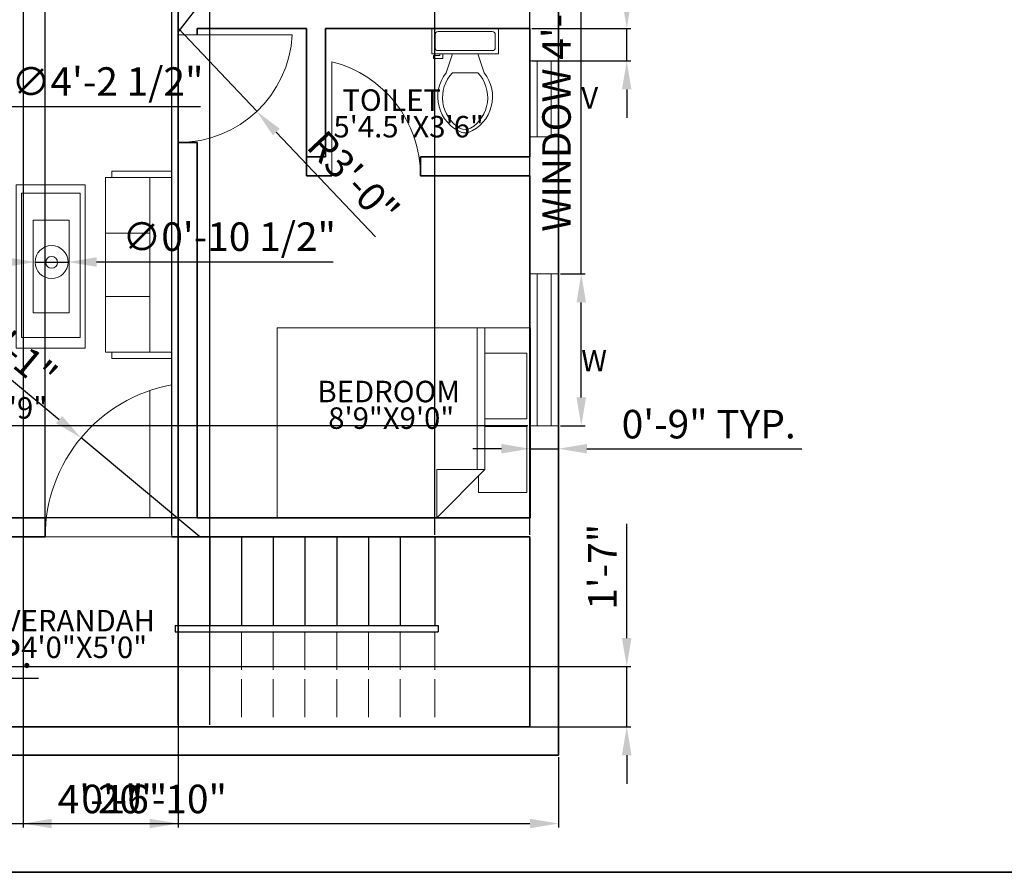
# Model space of a CAD drawing. Units: inches. Extents: x 1838 to 3181, y 1882 to 2430.
# Tile 2 of 4: x 2073 to 2384, y 1894 to 2163. Entities that reach past the tile are written whole.
import ezdxf

# ---------------------------------------------------------------- set-up
doc = ezdxf.new("R2010")
doc.units = ezdxf.units.IN
doc.linetypes.add('ACAD_ISO02W100', pattern=[15, 12, -3])
for name, color, linetype, lineweight in [('A-ANNO-TEXT', 7, 'Continuous', 18), ('A-ANNO-TTLB', 7, 'Continuous', 35), ('A-AREA-IDEN', 7, 'Continuous', 18), ('A-DOOR', 4, 'Continuous', 18), ('A-FLOR-FIXT', 9, 'Continuous', 18), ('A-FLOR-STRS', 7, 'Continuous', 25), ('A-FLOR-STRS-HIDN', 7, 'ACAD_ISO02W100', 18), ('A-FURN', 8, 'Continuous', 18), ('A-GLAZ', 11, 'Continuous', 18), ('A-WALL', 7, 'Continuous', 35), ('S-ANNO-DIMS', 2, 'Continuous', 18)]:
    doc.layers.add(name, color=color, linetype=linetype, lineweight=lineweight)
doc.styles.get("Standard").update_dxf_attribs({"font": 'arial.ttf'})
doc.dimstyles.new('ISO-25', dxfattribs={"dimtxt": 9, "dimasz": 9, "dimexe": 1.25, "dimexo": 0.625, "dimgap": 2, "dimtad": 1, "dimdec": 1, "dimlunit": 4, "dimtxsty": 'Standard', "dimcen": 2.5, "dimadec": 0, "dimazin": 0, "dimtfac": 1, "dimtdec": 1, "dimtmove": 0, "dimatfit": 3, "dimfxl": 1, "dimarcsym": 0})

# ---------------------------------------------------------------- blocks, each defined once
blk = doc.blocks.new('Bed - Queen')
for p, q in [((0, -80.00003), (0, 0)), ((0, 0), (59.99999, 0)), ((59.99999, 0), (59.99999, -80.00003)), ((7.99999, -1.2), (28.79998, -1.2)), ((7.99999, -14.4), (7.99999, -1.2)), ((28.79998, -1.2), (28.79998, -14.4)), ((31.19999, -1.2), (51.99999, -1.2)), ((31.19999, -14.4), (31.19999, -1.2)), ((51.99999, -1.2), (51.99999, -16.4)), ((0, -14.4), (44.8, -14.4)), ((59.99999, -29.6), (44.8, -14.4)), ((44.8, -14.4), (44.8, -29.6)), ((44.8, -16.8), (0, -16.8)), ((51.99999, -16.4), (46.79936, -16.4)), ((44.8, -29.6), (59.99999, -29.6)), ((59.99999, -80.00003), (0, -80.00003))]:
    blk.add_line(p, q)
blk = doc.blocks.new('Toilet - top')
for p, q in [((9.5, -6), (9.5, -2)), ((-10, -8.5), (-8, -8.5)), ((-10, -9.5), (-10, -8.5)), ((-8, -8.5), (-8, -8)), ((-7, -8), (-7, -9.5)), ((-4, -8), (-6, -14)), ((4, -8), (6, -14)), ((-7, -9.5), (-10, -9.5)), ((4, -14), (-4, -14))]:
    blk.add_line(p, q)
blk.add_lwpolyline([(10.5, -8), (10.5, 0), (-10.5, 0), (-10.5, -8)], close=True)
for points in [[(-9.5, -2), (-9.5, -6)], [(8.5, -1), (-8.5, -1)], [(-8.5, -7), (8.5, -7)]]:
    blk.add_lwpolyline(points)
for centre, radius, start, end in [((-8.62, -1.88), 0.884, 81.8699, 188.1301), ((8.62, -1.88), 0.884, 351.8699, 98.1301), ((-8.62, -6.12), 0.884, 171.8699, 278.1301), ((8.62, -6.12), 0.884, 261.8699, 8.1301), ((3.52, -21.58), 12.17, 141.4691, 247.9714), ((4.2, -21.82), 11.33, 136.3677, 238.9468), ((-3.52, -21.58), 12.17, 292.0284, 38.5307), ((-4.2, -21.82), 11.33, 301.053, 43.6321), ((0, -27.88), 4, 245.7318, 294.2682), ((0, -29), 4, 254.8605, 285.1395)]:
    blk.add_arc(centre, radius, start, end)
blk = doc.blocks.new('WIN-48')
for p, q in [((0, 48), (9, 48)), ((2.25, 48), (2.25, 0)), ((6.75, 48), (6.75, 0)), ((0, 0), (9, 0))]:
    blk.add_line(p, q)
blk = doc.blocks.new('VENT-24')
for p, q in [((0, 24), (9, 24)), ((2.25, 24), (2.25, 0)), ((6.75, 24), (6.75, 0)), ((0, 0), (9, 0))]:
    blk.add_line(p, q)
blk = doc.blocks.new('DOOR-SWING-36')
blk.add_line((0, 0), (36, 0))
blk.add_arc((0, -9.14), 37.14, 14.25, 90)
blk = doc.blocks.new('*D23')
at = {"layer": 'Defpoints', "color": 0, "transparency": 16777216}
for p in [(2243.53, 2082.46), (2250.73, 2082.46), (2243.53, 2034.46)]:
    blk.add_point(p, dxfattribs=at)
at = {"layer": 'S-ANNO-DIMS', "color": 0, "lineweight": -2, "transparency": 16777216}
for p, q in [((2250.73, 2082.46), (2250.73, 2209.34)), ((2244.16, 2082.46), (2251.98, 2082.46)), ((2250.73, 2043.46), (2250.73, 2073.46)), ((2244.16, 2034.46), (2251.98, 2034.46))]:
    blk.add_line(p, q, dxfattribs=at)
at = {"layer": 'S-ANNO-DIMS', "color": 0, "transparency": 16777216}
for points in [[(2249.23, 2073.46), (2252.23, 2073.46), (2250.73, 2082.46)], [(2249.23, 2043.46), (2252.23, 2043.46), (2250.73, 2034.46)]]:
    blk.add_solid(points, dxfattribs=at)
at = {"layer": 'S-ANNO-DIMS', "color": 0, "transparency": 16777216, "insert": (2244.08, 2150.4), "char_height": 9, "attachment_point": 5, "rotation": 90}
blk.add_mtext('WINDOW 4\'-0" TYP.', dxfattribs=at)
blk = doc.blocks.new('*D24')
at = {"layer": 'Defpoints', "color": 0, "transparency": 16777216}
for p in [(2234.53, 2034.46), (2243.53, 2034.46), (2243.53, 2027.26)]:
    blk.add_point(p, dxfattribs=at)
at = {"layer": 'S-ANNO-DIMS', "color": 0, "lineweight": -2, "transparency": 16777216}
for p, q in [((2234.53, 2033.83), (2234.53, 2026.01)), ((2243.53, 2033.83), (2243.53, 2026.01)), ((2225.53, 2027.26), (2216.53, 2027.26)), ((2234.53, 2027.26), (2243.53, 2027.26)), ((2252.53, 2027.26), (2320.39, 2027.26))]:
    blk.add_line(p, q, dxfattribs=at)
at = {"layer": 'S-ANNO-DIMS', "color": 0, "transparency": 16777216}
for points in [[(2225.53, 2028.76), (2225.53, 2025.76), (2234.53, 2027.26)], [(2252.53, 2028.76), (2252.53, 2025.76), (2243.53, 2027.26)]]:
    blk.add_solid(points, dxfattribs=at)
at = {"layer": 'S-ANNO-DIMS', "color": 0, "transparency": 16777216, "insert": (2290.96, 2033.85), "char_height": 9, "attachment_point": 5}
blk.add_mtext('0\'-9" TYP.', dxfattribs=at)
blk = doc.blocks.new('*D26')
at = {"layer": 'Defpoints', "color": 0, "transparency": 16777216}
for p in [(1993.53, 1958.46), (2002.53, 1958.46), (2002.53, 1954.86)]:
    blk.add_point(p, dxfattribs=at)
at = {"layer": 'S-ANNO-DIMS', "color": 0, "lineweight": -2, "transparency": 16777216}
for p, q in [((1984.53, 1954.86), (1975.53, 1954.86)), ((1993.53, 1957.83), (1993.53, 1953.61)), ((1993.53, 1954.86), (2002.53, 1954.86)), ((2002.53, 1957.83), (2002.53, 1953.61)), ((2011.53, 1954.86), (2079.39, 1954.86))]:
    blk.add_line(p, q, dxfattribs=at)
at = {"layer": 'S-ANNO-DIMS', "color": 0, "transparency": 16777216}
for points in [[(1984.53, 1956.36), (1984.53, 1953.36), (1993.53, 1954.86)], [(2011.53, 1956.36), (2011.53, 1953.36), (2002.53, 1954.86)]]:
    blk.add_solid(points, dxfattribs=at)
at = {"layer": 'S-ANNO-DIMS', "color": 0, "transparency": 16777216, "insert": (2049.96, 1961.45), "char_height": 9, "attachment_point": 5}
blk.add_mtext('0\'-9" TYP.', dxfattribs=at)
blk = doc.blocks.new('*D39')
at = {"layer": 'Defpoints', "color": 0, "transparency": 16777216}
for p in [(1993.53, 1930.46), (2243.53, 1930.46), (2243.53, 1908.91)]:
    blk.add_point(p, dxfattribs=at)
at = {"layer": 'S-ANNO-DIMS', "color": 0, "lineweight": -2, "transparency": 16777216}
for p, q in [((1993.53, 1929.83), (1993.53, 1907.66)), ((2243.53, 1929.83), (2243.53, 1907.66)), ((2002.53, 1908.91), (2234.53, 1908.91))]:
    blk.add_line(p, q, dxfattribs=at)
at = {"layer": 'S-ANNO-DIMS', "color": 0, "transparency": 16777216}
for points in [[(2002.53, 1910.41), (2002.53, 1907.41), (1993.53, 1908.91)], [(2234.53, 1910.41), (2234.53, 1907.41), (2243.53, 1908.91)]]:
    blk.add_solid(points, dxfattribs=at)
at = {"layer": 'S-ANNO-DIMS', "color": 0, "transparency": 16777216, "insert": (2118.53, 1915.5), "char_height": 9, "attachment_point": 5}
blk.add_mtext('20\'-10"', dxfattribs=at)
blk = doc.blocks.new('*D41')
at = {"layer": 'Defpoints', "color": 0, "transparency": 16777216}
for p in [(2002.53, 1958.46), (2265.08, 1958.46), (2002.53, 1939.46)]:
    blk.add_point(p, dxfattribs=at)
at = {"layer": 'S-ANNO-DIMS', "color": 0, "lineweight": -2, "transparency": 16777216}
for p, q in [((2265.08, 1967.46), (2265.08, 2003.53)), ((2003.16, 1958.46), (2266.33, 1958.46)), ((2265.08, 1939.46), (2265.08, 1958.46)), ((2003.16, 1939.46), (2266.33, 1939.46)), ((2265.08, 1930.46), (2265.08, 1921.46))]:
    blk.add_line(p, q, dxfattribs=at)
at = {"layer": 'S-ANNO-DIMS', "color": 0, "transparency": 16777216}
for points in [[(2263.58, 1967.46), (2266.58, 1967.46), (2265.08, 1958.46)], [(2263.58, 1930.46), (2266.58, 1930.46), (2265.08, 1939.46)]]:
    blk.add_solid(points, dxfattribs=at)
at = {"layer": 'S-ANNO-DIMS', "color": 0, "transparency": 16777216, "insert": (2258.57, 1989.99), "char_height": 9, "attachment_point": 5, "rotation": 90}
blk.add_mtext('1\'-7"', dxfattribs=at)
blk = doc.blocks.new('*D45')
at = {"layer": 'Defpoints', "color": 0, "transparency": 16777216}
for p in [(1971.98, 2034.46), (2234.53, 2034.46), (2234.53, 2005.46)]:
    blk.add_point(p, dxfattribs=at)
at = {"layer": 'S-ANNO-DIMS', "color": 0, "lineweight": -2, "transparency": 16777216}
for p, q in [((2233.91, 2034.46), (1970.73, 2034.46)), ((1971.98, 2014.46), (1971.98, 2025.46)), ((2233.91, 2005.46), (1970.73, 2005.46))]:
    blk.add_line(p, q, dxfattribs=at)
at = {"layer": 'S-ANNO-DIMS', "color": 0, "transparency": 16777216}
for points in [[(1970.48, 2025.46), (1973.48, 2025.46), (1971.98, 2034.46)], [(1970.48, 2014.46), (1973.48, 2014.46), (1971.98, 2005.46)]]:
    blk.add_solid(points, dxfattribs=at)
at = {"layer": 'S-ANNO-DIMS', "color": 0, "transparency": 16777216, "insert": (1965.39, 2019.96), "char_height": 9, "attachment_point": 5, "rotation": 90}
blk.add_mtext('2\'-5"', dxfattribs=at)
blk = doc.blocks.new('*D46')
at = {"layer": 'Defpoints', "color": 0, "transparency": 16777216}
for p in [(2234.53, 2159.96), (2265.08, 2159.96), (2234.53, 2149.73)]:
    blk.add_point(p, dxfattribs=at)
at = {"layer": 'S-ANNO-DIMS', "color": 0, "lineweight": -2, "transparency": 16777216}
for p, q in [((2265.08, 2168.96), (2265.08, 2212.87)), ((2235.16, 2159.96), (2266.33, 2159.96)), ((2265.08, 2149.73), (2265.08, 2159.96)), ((2235.16, 2149.73), (2266.33, 2149.73)), ((2265.08, 2140.73), (2265.08, 2131.73))]:
    blk.add_line(p, q, dxfattribs=at)
at = {"layer": 'S-ANNO-DIMS', "color": 0, "transparency": 16777216}
for points in [[(2263.58, 2168.96), (2266.58, 2168.96), (2265.08, 2159.96)], [(2263.58, 2140.73), (2266.58, 2140.73), (2265.08, 2149.73)]]:
    blk.add_solid(points, dxfattribs=at)
at = {"layer": 'S-ANNO-DIMS', "color": 0, "transparency": 16777216, "insert": (2258.49, 2195.41), "char_height": 9, "attachment_point": 5, "rotation": 90}
blk.add_mtext('0\'-10"', dxfattribs=at)
blk = doc.blocks.new('*D49')
at = {"layer": 'Defpoints', "color": 0, "transparency": 16777216}
for p in [(2133.53, 2362.82), (2123.53, 1939.46), (2133.53, 1939.46)]:
    blk.add_point(p, dxfattribs=at)
at = {"layer": 'S-ANNO-DIMS', "color": 0, "lineweight": -2, "transparency": 16777216}
for p, q in [((2114.53, 2362.82), (2105.53, 2362.82)), ((2123.53, 1940.08), (2123.53, 2364.07)), ((2123.53, 2362.82), (2133.53, 2362.82)), ((2133.53, 1940.08), (2133.53, 2364.07)), ((2142.53, 2362.82), (2186.45, 2362.82))]:
    blk.add_line(p, q, dxfattribs=at)
at = {"layer": 'S-ANNO-DIMS', "color": 0, "transparency": 16777216}
for points in [[(2114.53, 2364.32), (2114.53, 2361.32), (2123.53, 2362.82)], [(2142.53, 2364.32), (2142.53, 2361.32), (2133.53, 2362.82)]]:
    blk.add_solid(points, dxfattribs=at)
at = {"layer": 'S-ANNO-DIMS', "color": 0, "transparency": 16777216, "insert": (2168.99, 2369.41), "char_height": 9, "attachment_point": 5}
blk.add_mtext('0\'-10"', dxfattribs=at)
blk = doc.blocks.new('*D50')
at = {"layer": 'Defpoints', "color": 0, "transparency": 16777216}
for p in [(2204.53, 2362.82), (2123.53, 1999.46), (2204.53, 1999.46)]:
    blk.add_point(p, dxfattribs=at)
at = {"layer": 'S-ANNO-DIMS', "color": 0, "lineweight": -2, "transparency": 16777216}
for p, q in [((2123.53, 2000.08), (2123.53, 2364.07)), ((2132.53, 2362.82), (2195.53, 2362.82)), ((2204.53, 2000.08), (2204.53, 2364.07))]:
    blk.add_line(p, q, dxfattribs=at)
at = {"layer": 'S-ANNO-DIMS', "color": 0, "transparency": 16777216}
for points in [[(2132.53, 2364.32), (2132.53, 2361.32), (2123.53, 2362.82)], [(2195.53, 2364.32), (2195.53, 2361.32), (2204.53, 2362.82)]]:
    blk.add_solid(points, dxfattribs=at)
at = {"layer": 'S-ANNO-DIMS', "color": 0, "transparency": 16777216, "insert": (2164.03, 2369.41), "char_height": 9, "attachment_point": 5}
blk.add_mtext('6\'-9"', dxfattribs=at)
blk = doc.blocks.new('*D51')
at = {"layer": 'Defpoints', "color": 0, "transparency": 16777216}
for p in [(2234.53, 2362.82), (2204.53, 1999.46), (2234.53, 1999.46)]:
    blk.add_point(p, dxfattribs=at)
at = {"layer": 'S-ANNO-DIMS', "color": 0, "lineweight": -2, "transparency": 16777216}
for p, q in [((2204.53, 2000.08), (2204.53, 2364.07)), ((2213.53, 2362.82), (2225.53, 2362.82)), ((2234.53, 2000.08), (2234.53, 2364.07))]:
    blk.add_line(p, q, dxfattribs=at)
at = {"layer": 'S-ANNO-DIMS', "color": 0, "transparency": 16777216}
for points in [[(2213.53, 2364.32), (2213.53, 2361.32), (2204.53, 2362.82)], [(2225.53, 2364.32), (2225.53, 2361.32), (2234.53, 2362.82)]]:
    blk.add_solid(points, dxfattribs=at)
at = {"layer": 'S-ANNO-DIMS', "color": 0, "transparency": 16777216, "insert": (2219.53, 2369.41), "char_height": 9, "attachment_point": 5}
blk.add_mtext('2\'-6"', dxfattribs=at)
blk = doc.blocks.new('*D53')
at = {"layer": 'Defpoints', "color": 0, "transparency": 16777216}
for p in [(2121.53, 2362.82), (2081.53, 1999.46), (2121.53, 1999.46)]:
    blk.add_point(p, dxfattribs=at)
at = {"layer": 'S-ANNO-DIMS', "color": 0, "lineweight": -2, "transparency": 16777216}
for p, q in [((2081.53, 2000.08), (2081.53, 2364.07)), ((2090.53, 2362.82), (2112.53, 2362.82)), ((2121.53, 2000.08), (2121.53, 2364.07))]:
    blk.add_line(p, q, dxfattribs=at)
at = {"layer": 'S-ANNO-DIMS', "color": 0, "transparency": 16777216}
for points in [[(2090.53, 2364.32), (2090.53, 2361.32), (2081.53, 2362.82)], [(2112.53, 2364.32), (2112.53, 2361.32), (2121.53, 2362.82)]]:
    blk.add_solid(points, dxfattribs=at)
at = {"layer": 'S-ANNO-DIMS', "color": 0, "transparency": 16777216, "insert": (2101.53, 2369.42), "char_height": 9, "attachment_point": 5}
blk.add_mtext('3\'-4"', dxfattribs=at)
blk = doc.blocks.new('*D55')
at = {"layer": 'Defpoints', "color": 0, "transparency": 16777216}
for p in [(2068.53, 2194.46), (2074.53, 2194.46), (2074.53, 1908.91)]:
    blk.add_point(p, dxfattribs=at)
at = {"layer": 'S-ANNO-DIMS', "color": 0, "lineweight": -2, "transparency": 16777216}
for p, q in [((2068.53, 2193.83), (2068.53, 1907.66)), ((2074.53, 2193.83), (2074.53, 1907.66)), ((2059.53, 1908.91), (2050.53, 1908.91)), ((2068.53, 1908.91), (2074.53, 1908.91)), ((2083.53, 1908.91), (2120.46, 1908.91))]:
    blk.add_line(p, q, dxfattribs=at)
at = {"layer": 'S-ANNO-DIMS', "color": 0, "transparency": 16777216}
for points in [[(2059.53, 1910.41), (2059.53, 1907.41), (2068.53, 1908.91)], [(2083.53, 1910.41), (2083.53, 1907.41), (2074.53, 1908.91)]]:
    blk.add_solid(points, dxfattribs=at)
at = {"layer": 'S-ANNO-DIMS', "color": 0, "transparency": 16777216, "insert": (2106.5, 1915.5), "char_height": 9, "attachment_point": 5}
blk.add_mtext('0\'-6"', dxfattribs=at)
blk = doc.blocks.new('*D56')
at = {"layer": 'Defpoints', "color": 0, "transparency": 16777216}
for p in [(2074.53, 2218.46), (2123.53, 2218.46), (2123.53, 1908.91)]:
    blk.add_point(p, dxfattribs=at)
at = {"layer": 'S-ANNO-DIMS', "color": 0, "lineweight": -2, "transparency": 16777216}
for p, q in [((2074.53, 2217.83), (2074.53, 1907.66)), ((2123.53, 2217.83), (2123.53, 1907.66)), ((2083.53, 1908.91), (2114.53, 1908.91))]:
    blk.add_line(p, q, dxfattribs=at)
at = {"layer": 'S-ANNO-DIMS', "color": 0, "transparency": 16777216}
for points in [[(2083.53, 1910.41), (2083.53, 1907.41), (2074.53, 1908.91)], [(2114.53, 1910.41), (2114.53, 1907.41), (2123.53, 1908.91)]]:
    blk.add_solid(points, dxfattribs=at)
at = {"layer": 'S-ANNO-DIMS', "color": 0, "transparency": 16777216, "insert": (2099.03, 1915.42), "char_height": 9, "attachment_point": 5}
blk.add_mtext('4\'-1"', dxfattribs=at)
blk = doc.blocks.new('*D68')
at = {"layer": 'Defpoints', "color": 0, "transparency": 16777216}
for p in [(2003.51, 2135.2), (2053.84, 2135.2)]:
    blk.add_point(p, dxfattribs=at)
at = {"layer": 'S-ANNO-DIMS', "color": 0, "lineweight": -2, "transparency": 16777216}
for p, q in [((1994.51, 2135.2), (1985.51, 2135.2)), ((2003.51, 2135.2), (2053.84, 2135.2)), ((2130.53, 2135.2), (2062.84, 2135.2))]:
    blk.add_line(p, q, dxfattribs=at)
at = {"layer": 'S-ANNO-DIMS', "color": 0, "transparency": 16777216}
for points in [[(1994.51, 2136.7), (1994.51, 2133.7), (2003.51, 2135.2)], [(2062.84, 2136.7), (2062.84, 2133.7), (2053.84, 2135.2)]]:
    blk.add_solid(points, dxfattribs=at)
at = {"layer": 'S-ANNO-DIMS', "color": 0, "transparency": 16777216, "insert": (2101.19, 2142.04), "char_height": 9, "attachment_point": 5, "rotation": 359.9991}
blk.add_mtext('∅4\'-2 1/2"', dxfattribs=at)
blk = doc.blocks.new('*D69')
at = {"layer": 'Defpoints', "color": 0, "transparency": 16777216}
for p in [(2078.35, 2086.21), (2088.77, 2086.21)]:
    blk.add_point(p, dxfattribs=at)
at = {"layer": 'S-ANNO-DIMS', "color": 0, "lineweight": -2, "transparency": 16777216}
for p, q in [((2069.35, 2086.21), (2060.35, 2086.21)), ((2078.35, 2086.21), (2088.77, 2086.21)), ((2172.45, 2086.22), (2097.77, 2086.21))]:
    blk.add_line(p, q, dxfattribs=at)
at = {"layer": 'S-ANNO-DIMS', "color": 0, "transparency": 16777216}
for points in [[(2069.35, 2087.71), (2069.35, 2084.71), (2078.35, 2086.21)], [(2097.77, 2087.71), (2097.77, 2084.71), (2088.77, 2086.21)]]:
    blk.add_solid(points, dxfattribs=at)
at = {"layer": 'S-ANNO-DIMS', "color": 0, "transparency": 16777216, "insert": (2139.61, 2093.06), "char_height": 9, "attachment_point": 5, "rotation": 0.0024}
blk.add_mtext('∅0\'-10 1/2"', dxfattribs=at)
blk = doc.blocks.new('*D70')
at = {"layer": 'Defpoints', "color": 0, "transparency": 16777216}
for p in [(2092.84, 2030.7), (2130.33, 1999.46)]:
    blk.add_point(p, dxfattribs=at)
at = {"layer": 'S-ANNO-DIMS', "color": 0, "lineweight": -2, "transparency": 16777216}
for p, q in [((2050.95, 2065.61), (2085.93, 2036.46)), ((2130.33, 1999.46), (2092.84, 2030.7))]:
    blk.add_line(p, q, dxfattribs=at)
at = {"layer": 'S-ANNO-DIMS', "color": 0, "transparency": 16777216}
blk.add_solid([(2086.89, 2037.61), (2084.97, 2035.31), (2092.84, 2030.7)], dxfattribs=at)
at = {"layer": 'S-ANNO-DIMS', "color": 0, "transparency": 16777216, "insert": (2069.16, 2058.92), "char_height": 9, "attachment_point": 5, "rotation": 320.1941}
blk.add_mtext('R4\'-1"', dxfattribs=at)
blk = doc.blocks.new('*D72')
at = {"layer": 'Defpoints', "color": 0, "transparency": 16777216}
for p in [(2146.34, 2188.13), (2123.53, 2158.81)]:
    blk.add_point(p, dxfattribs=at)
at = {"layer": 'S-ANNO-DIMS', "color": 0, "lineweight": -2, "transparency": 16777216}
for p, q in [((2179.82, 2231.18), (2151.86, 2195.24)), ((2123.53, 2158.81), (2146.34, 2188.13))]:
    blk.add_line(p, q, dxfattribs=at)
at = {"layer": 'S-ANNO-DIMS', "color": 0, "transparency": 16777216}
blk.add_solid([(2150.68, 2196.16), (2153.05, 2194.32), (2146.34, 2188.13)], dxfattribs=at)
at = {"layer": 'S-ANNO-DIMS', "color": 0, "transparency": 16777216, "insert": (2163.4, 2220.81), "char_height": 9, "attachment_point": 5, "rotation": 52.1256}
blk.add_mtext('R3\'-1"', dxfattribs=at)
blk = doc.blocks.new('*D73')
at = {"layer": 'Defpoints', "color": 0, "transparency": 16777216}
for p in [(2123.53, 2160.01), (2148.29, 2133.8)]:
    blk.add_point(p, dxfattribs=at)
at = {"layer": 'S-ANNO-DIMS', "color": 0, "lineweight": -2, "transparency": 16777216}
for p, q in [((2123.53, 2160.01), (2148.29, 2133.8)), ((2185.74, 2094.15), (2154.47, 2127.26))]:
    blk.add_line(p, q, dxfattribs=at)
at = {"layer": 'S-ANNO-DIMS', "color": 0, "transparency": 16777216}
blk.add_solid([(2155.56, 2128.29), (2153.38, 2126.23), (2148.29, 2133.8)], dxfattribs=at)
at = {"layer": 'S-ANNO-DIMS', "color": 0, "transparency": 16777216, "insert": (2177.99, 2111.96), "char_height": 9, "attachment_point": 5, "rotation": 313.3644}
blk.add_mtext('R3\'-0"', dxfattribs=at)

msp = doc.modelspace()

# ---------------------------------------------------------------- linework, layer by layer
at = {"layer": 'A-ANNO-TTLB'}
msp.add_lwpolyline([(1905.37, 2389.23), (3180.85, 2389.23), (3180.85, 1893.51), (1905.37, 1893.51)], close=True, dxfattribs=at)
at = {"layer": 'A-DOOR'}
for p, q in [((2123.53, 2157.96), (2159.53, 2157.96)), ((2114.53, 2045.63), (2114.53, 2005.46)), ((2121.53, 2047.46), (2121.53, 1999.46)), ((2121.53, 2047.46), (2121.53, 2005.46)), ((2081.53, 1999.46), (2121.53, 1999.46))]:
    msp.add_line(p, q, dxfattribs=at)
for centre, radius, start, end in [((2123.53, 2160.01), 36.06, 270, 356.7268), ((2130.33, 1999.46), 48.8, 100.3889, 180)]:
    msp.add_arc(centre, radius, start, end, dxfattribs=at)
at = {"layer": 'A-FLOR-STRS'}
for p, q in [((2123.53, 1999.46), (2123.53, 1971.46)), ((2133.53, 1999.46), (2133.53, 1971.46)), ((2143.53, 1999.46), (2143.53, 1971.46)), ((2153.53, 1999.46), (2153.53, 1971.46)), ((2163.53, 1999.46), (2163.53, 1971.46)), ((2173.53, 1999.46), (2173.53, 1971.46)), ((2183.53, 1999.46), (2183.53, 1971.46)), ((2193.53, 1999.46), (2193.53, 1971.46)), ((2204.53, 1999.46), (2204.53, 1971.46)), ((2122.53, 1971.46), (2205.53, 1971.46)), ((2122.53, 1971.46), (2122.53, 1969.46)), ((2205.53, 1971.46), (2205.53, 1969.46)), ((2122.53, 1969.46), (2205.53, 1969.46))]:
    msp.add_line(p, q, dxfattribs=at)
at = {"layer": 'A-FLOR-STRS-HIDN'}
for p, q in [((2123.53, 1969.46), (2123.53, 1939.46)), ((2133.53, 1969.46), (2133.53, 1939.46)), ((2143.53, 1969.46), (2143.53, 1939.46)), ((2153.53, 1969.46), (2153.53, 1939.46)), ((2163.53, 1969.46), (2163.53, 1939.46)), ((2173.53, 1969.46), (2173.53, 1939.46)), ((2183.53, 1969.46), (2183.53, 1939.46)), ((2193.53, 1969.46), (2193.53, 1939.46)), ((2204.53, 1969.46), (2204.53, 1939.46))]:
    msp.add_line(p, q, dxfattribs=at)
at = {"layer": 'A-FURN'}
for p, q in [((2102.53, 2114.94), (2102.53, 2112.94)), ((2121.53, 2114.94), (2102.53, 2114.94)), ((2121.53, 2114.94), (2121.53, 2055.71)), ((2121.53, 2112.94), (2100.53, 2112.94)), ((2100.53, 2112.94), (2100.53, 2057.71)), ((2114.53, 2112.94), (2114.53, 2057.71)), ((2114.53, 2095.34), (2100.53, 2095.34)), ((2100.53, 2075.31), (2114.53, 2075.31)), ((2100.53, 2057.71), (2121.53, 2057.71)), ((2102.53, 2057.71), (2102.53, 2055.71)), ((2102.53, 2055.71), (2121.53, 2055.71))]:
    msp.add_line(p, q, dxfattribs=at)
for points in [[(2072.38, 2110.61), (2094.15, 2110.61), (2094.15, 2059.05), (2072.38, 2059.05)], [(2074.1, 2107.93), (2092.53, 2107.93), (2092.53, 2062.39), (2074.1, 2062.39)], [(2077.78, 2099.42), (2089.11, 2099.42), (2089.11, 2070.17), (2077.78, 2070.17)]]:
    msp.add_lwpolyline(points, close=True, dxfattribs=at)
for centre, radius in [((2083.56, 2086.21), 5.21), ((2083.56, 2086.09), 1.86)]:
    msp.add_circle(centre, radius, dxfattribs=at)
at = {"layer": 'A-WALL'}
for p, q in [((2243.53, 2293.46), (2243.53, 1930.46)), ((2123.53, 2167.96), (2123.53, 2157.96)), ((2129.53, 2159.96), (2164.03, 2159.96)), ((2129.53, 2159.96), (2129.53, 2157.96)), ((2164.03, 2159.96), (2164.03, 2113.46)), ((2170.03, 2159.96), (2170.03, 2119.46)), ((2170.03, 2159.96), (2234.53, 2159.96)), ((2234.53, 2159.96), (2234.53, 2119.46)), ((2123.53, 2123.96), (2129.53, 2123.96)), ((2123.53, 2123.96), (2123.53, 2005.46)), ((2129.53, 2123.96), (2129.53, 2005.46)), ((2164.03, 2119.46), (2170.03, 2119.46)), ((2200.03, 2119.46), (2234.53, 2119.46)), ((2200.03, 2119.46), (2200.03, 2113.46)), ((2164.03, 2113.46), (2172.03, 2113.46)), ((2200.03, 2113.46), (2234.53, 2113.46)), ((2234.53, 2113.46), (2234.53, 2005.46)), ((2042.53, 2005.46), (2081.53, 2005.46)), ((2081.53, 2005.46), (2081.53, 1999.46)), ((2121.53, 2005.46), (2123.53, 2005.46)), ((2129.53, 2005.46), (2234.53, 2005.46)), ((2068.53, 1999.46), (2081.53, 1999.46)), ((2121.53, 1999.46), (2234.53, 1999.46)), ((2234.53, 1999.46), (2234.53, 1939.46)), ((2068.53, 1939.46), (2234.53, 1939.46)), ((1993.53, 1930.46), (2243.53, 1930.46))]:
    msp.add_line(p, q, dxfattribs=at)

# ---------------------------------------------------------------- block references
at = {"layer": 'A-DOOR', "extrusion": (0, 0, -1), "zscale": -1, "rotation": 89.99999999999969}
msp.add_blockref('DOOR-SWING-36', (-2172.03, 2113.46), dxfattribs=at)
at = {"layer": 'A-FLOR-FIXT'}
msp.add_blockref('Toilet - top', (2214.08, 2159.96), dxfattribs=at)
at = {"layer": 'A-FURN', "rotation": 270}
msp.add_blockref('Bed - Queen', (2234.7, 2065.47), dxfattribs=at)
at = {"layer": 'A-GLAZ'}
for name, p in [('VENT-24', (2234.53, 2125.73)), ('WIN-48', (2234.53, 2034.46))]:
    msp.add_blockref(name, p, dxfattribs=at)

# ---------------------------------------------------------------- texts
at = {"layer": 'A-ANNO-TEXT'}
for s, p in [('V', (2250.72, 2134.67)), ('W', (2250.72, 2051.7))]:
    msp.add_text(s, height=6.78, dxfattribs=at).set_placement(p)
at = {"layer": 'A-AREA-IDEN'}
for s, height, p in [(' TOILET', 6.784, (2173.25, 2133.95)), (' 5\'4.5"X3\'6"', 6.7841, (2170.44, 2125.55)), ('BEDROOM', 6.784, (2167.45, 2041.93)), ('    9\'4.5"X15\'9"', 6.7841, (2021.24, 2036.76)), ('   8\'9"X9\'0"', 6.7841, (2164.64, 2033.53)), ('VERANDAH', 6.784, (2068.46, 1969.58)), ('    4\'0"X5\'0"', 6.7841, (2065.65, 1961.17))]:
    msp.add_text(s, height=height, dxfattribs=at).set_placement(p)

# ---------------------------------------------------------------- dimensions: what is measured, and where the dimension line sits
at = {"layer": 'S-ANNO-DIMS'}
for base, p1, p2, picture, middle in [((2121.53, 2362.82), (2081.53, 1999.46), (2121.53, 1999.46), '*D53', (2101.53, 2369.42)), ((2133.53, 2362.82), (2123.53, 1939.46), (2133.53, 1939.46), '*D49', (2168.99, 2369.41)), ((2204.53, 2362.82), (2123.53, 1999.46), (2204.53, 1999.46), '*D50', (2164.03, 2369.41)), ((2234.53, 2362.82), (2204.53, 1999.46), (2234.53, 1999.46), '*D51', (2219.53, 2369.41)), ((2123.53, 1908.91), (2074.53, 2218.46), (2123.53, 2218.46), '*D56', (2099.03, 1915.42)), ((2074.53, 1908.91), (2068.53, 2194.46), (2074.53, 2194.46), '*D55', (2106.5, 1915.5)), ((2243.53, 1908.91), (1993.53, 1930.46), (2243.53, 1930.46), '*D39', (2118.53, 1915.5))]:
    dim = msp.add_linear_dim(base=base, p1=p1, p2=p2, dimstyle='ISO-25', override={"dimdec": 1, "dimlfac": 1, "dimrnd": 0, "dimzin": 1, "dimdsep": 46, "dimlunit": 4, "dimfrac": 2}, dxfattribs=at)
    dim.commit()
    dim.dimension.update_dxf_attribs({"geometry": picture, "text_midpoint": middle})
for center, mpoint, picture, middle in [((2123.53, 2158.81), (2146.34, 2188.13), '*D72', (2163.4, 2220.81)), ((2123.53, 2160.01), (2148.29, 2133.8), '*D73', (2177.99, 2111.96)), ((2130.33, 1999.46), (2092.84, 2030.7), '*D70', (2069.16, 2058.92))]:
    dim = msp.add_radius_dim(center=center, mpoint=mpoint, dimstyle='ISO-25', override={"dimdec": 1, "dimlfac": 1, "dimrnd": 0, "dimzin": 1, "dimdsep": 46, "dimlunit": 4, "dimfrac": 2}, dxfattribs=at)
    dim.commit()
    dim.dimension.update_dxf_attribs({"geometry": picture, "text_midpoint": middle})
for base, p1, p2, picture, middle in [((2265.08, 2159.96), (2234.53, 2149.73), (2234.53, 2159.96), '*D46', (2258.49, 2195.41)), ((1971.98, 2034.46), (2234.53, 2005.46), (2234.53, 2034.46), '*D45', (1965.39, 2019.96)), ((2265.08, 1958.46), (2002.53, 1939.46), (2002.53, 1958.46), '*D41', (2258.57, 1989.99))]:
    dim = msp.add_linear_dim(base=base, p1=p1, p2=p2, angle=90, dimstyle='ISO-25', override={"dimdec": 1, "dimlfac": 1, "dimrnd": 0, "dimzin": 1, "dimdsep": 46, "dimlunit": 4, "dimfrac": 2}, dxfattribs=at)
    dim.commit()
    dim.dimension.update_dxf_attribs({"geometry": picture, "text_midpoint": middle})
dim = msp.add_linear_dim(base=(2250.73, 2082.46), p1=(2243.53, 2034.46), p2=(2243.53, 2082.46), angle=90, text='WINDOW <> TYP.', dimstyle='ISO-25', override={"dimdec": 1, "dimlfac": 1, "dimrnd": 0, "dimzin": 1, "dimdsep": 46, "dimlunit": 4, "dimfrac": 2}, dxfattribs=at)
dim.commit()
dim.dimension.update_dxf_attribs({"geometry": '*D23', "text_midpoint": (2244.08, 2150.4)})
for p1, p2, picture, middle in [((2003.51, 2135.2), (2053.84, 2135.2), '*D68', (2101.19, 2135.2)), ((2078.35, 2086.21), (2088.77, 2086.21), '*D69', (2139.61, 2086.22))]:
    dim = msp.add_diameter_dim_2p(p1=p1, p2=p2, dimstyle='ISO-25', override={"dimdec": 1, "dimlfac": 1, "dimrnd": 0, "dimzin": 1, "dimdsep": 46, "dimlunit": 4, "dimfrac": 2}, dxfattribs=at)
    dim.commit()
    dim.dimension.update_dxf_attribs({"geometry": picture, "text_midpoint": middle})
for base, p1, p2, picture, middle in [((2243.53, 2027.26), (2234.53, 2034.46), (2243.53, 2034.46), '*D24', (2290.96, 2033.85)), ((2002.53, 1954.86), (1993.53, 1958.46), (2002.53, 1958.46), '*D26', (2049.96, 1961.45))]:
    dim = msp.add_linear_dim(base=base, p1=p1, p2=p2, text='<> TYP.', dimstyle='ISO-25', override={"dimdec": 1, "dimlfac": 1, "dimrnd": 0, "dimzin": 1, "dimdsep": 46, "dimlunit": 4, "dimfrac": 2}, dxfattribs=at)
    dim.commit()
    dim.dimension.update_dxf_attribs({"geometry": picture, "text_midpoint": middle})

doc.saveas('drawing.dxf')
